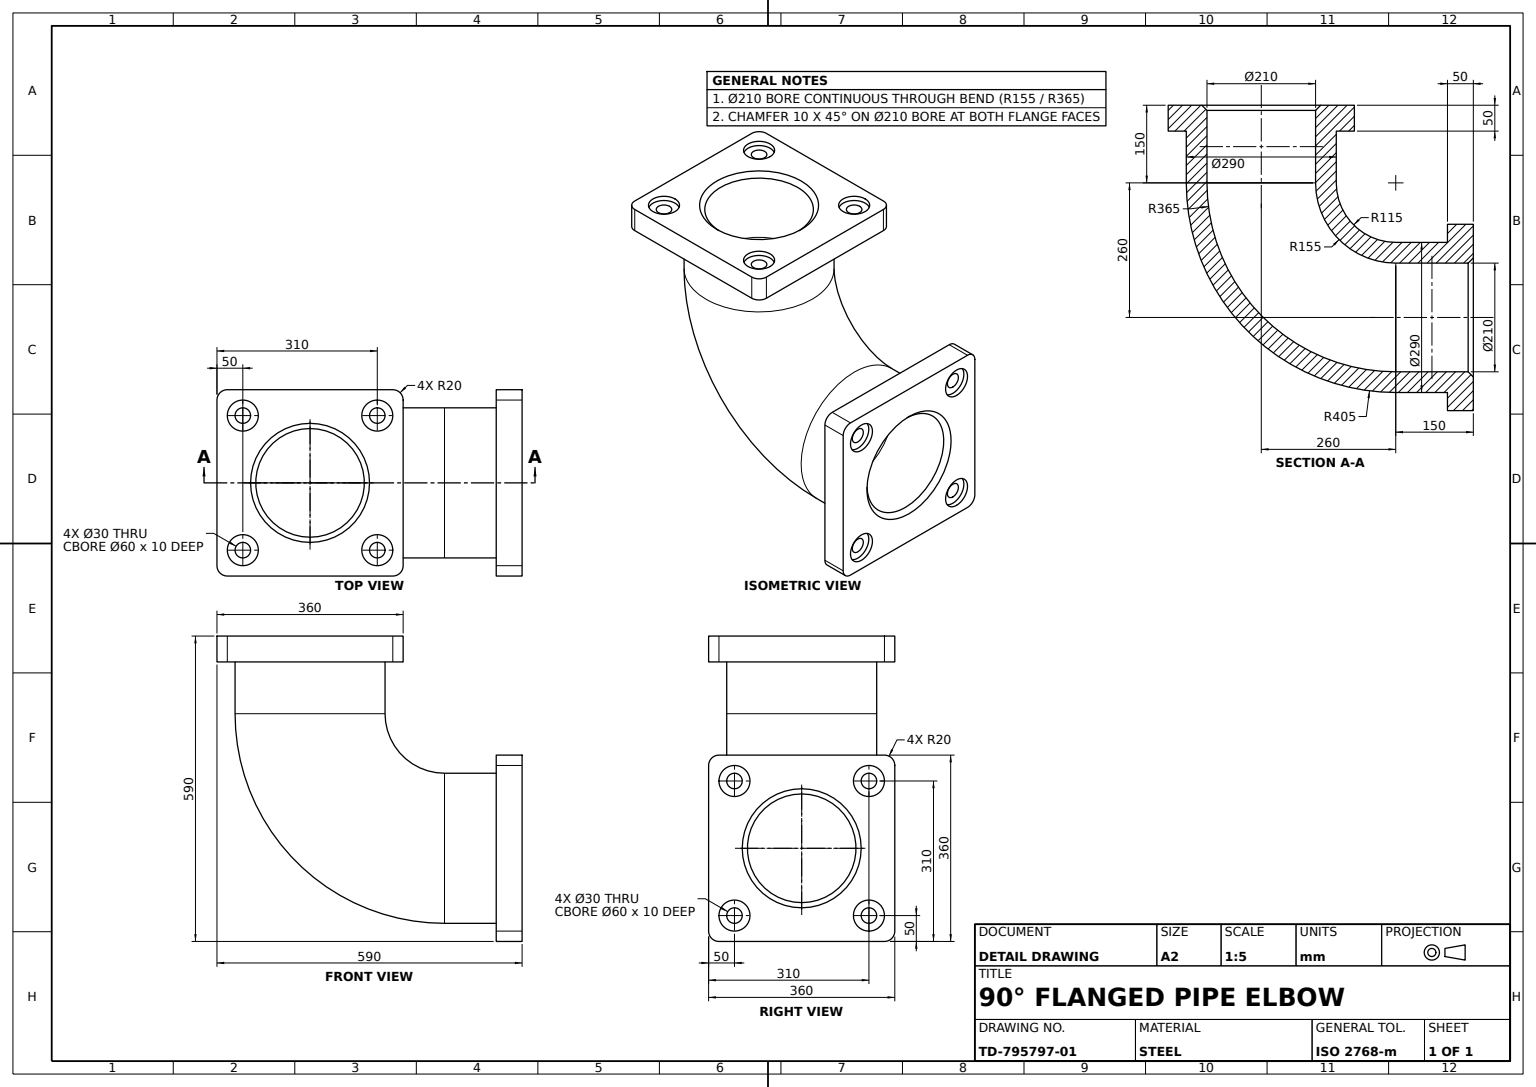
from build123d import *

# Parameters (mm, degrees)
PIPE_PROFILE_SKETCH_290_R           = 145
PIPE_PROFILE_SKETCH_290_R_2         = 105
FLANGE_START                        = -50
FLANGE_A_SKETCH_360X360_W           = 360
FLANGE_A_SKETCH_360X360_H           = 360
FLANGE_A_SKETCH_360X360_R           = 145
FLANGE_A_360X360X50_DEPTH           = 50
FLANGE_A_CORNER_FILLETS_R20_R       = 20
FLANGE_B_SKETCH_360X360_W           = 360
FLANGE_B_SKETCH_360X360_H           = 360
FLANGE_B_SKETCH_360X360_R           = 145
FLANGE_B_360X360X50_DEPTH           = 50
FLANGE_B_CORNER_FILLETS_R20_R       = 20
FLANGE_A_COUNTERBORE_SKETCH_60_R    = 30
FLANGE_A_COUNTERBORE_60X10_DEPTH    = 10
FLANGE_A_BOLT_HOLE_30_REACH         = 734.735
FLANGE_A_BOLT_HOLE_SKETCH_30_R      = 15
FLANGE_A_BOLT_HOLE_PATTERN_4X_COUNT = 4
FLANGE_B_COUNTERBORE_SKETCH_60_R    = 30
FLANGE_B_COUNTERBORE_60X10_DEPTH    = 10
FLANGE_B_BOLT_HOLE_30_REACH         = 848.699
FLANGE_B_BOLT_HOLE_SKETCH_30_R      = 15
FLANGE_B_BOLT_HOLE_PATTERN_4X_COUNT = 4
PIPE_EDGE_CHAMFER_10X45DEG_SIZE     = 10


with BuildPart() as part:
    # Elbow Pipe Sweep Wall 40: sweep along a path in Elbow Path Sketch
    with BuildLine(Plane.XY) as elbow_pipe_sweep_wall_40_path:
        Line((0, 0), (-150, 0))
        ThreePointArc((-150, 0), (-333.847763109, 76.152236891), (-410, 260))
        Line((-410, 260), (-410, 410))
    # Pipe Profile Sketch Ø290 → Elbow Pipe Sweep Wall 40 (sweep)
    with BuildSketch(Plane(origin=(0, 0, 0), x_dir=(0, 0, -1), z_dir=(1, 0, 0))):
        Circle(PIPE_PROFILE_SKETCH_290_R)
        Circle(PIPE_PROFILE_SKETCH_290_R_2, mode=Mode.SUBTRACT)
    sweep(path=elbow_pipe_sweep_wall_40_path.line)

    # Flange A Sketch 360x360 → Flange A 360x360x50 (add)
    with BuildSketch(Plane(origin=(0, 0, 0), x_dir=(0, 0, -1), z_dir=(1, 0, 0)).offset(FLANGE_START)):
        Rectangle(FLANGE_A_SKETCH_360X360_W, FLANGE_A_SKETCH_360X360_H)
        with Locations(Location((0, 0, 0), (0, 0, 270))):
            Circle(FLANGE_A_SKETCH_360X360_R, mode=Mode.SUBTRACT)
    extrude(amount=FLANGE_A_360X360X50_DEPTH)

    # Flange A Corner Fillets R20
    flange_a_corner_fillets_r20_edges = [part.edges().sort_by_distance(p)[0] for p in [
        (-25, 180, -180),
        (-25, -180, -180),
        (-25, -180, 180),
        (-25, 180, 180),
    ]]
    fillet(flange_a_corner_fillets_r20_edges, radius=FLANGE_A_CORNER_FILLETS_R20_R)

    # Flange B Sketch 360x360 → Flange B 360x360x50 (add)
    with BuildSketch(Plane(origin=(0, 410, 0), x_dir=(1, 0, 0), z_dir=(0, 1, 0))):
        with Locations((-410, 0)):
            Rectangle(FLANGE_B_SKETCH_360X360_W, FLANGE_B_SKETCH_360X360_H)
        with Locations(Location((-410, 0, 0), (0, 0, 180))):
            Circle(FLANGE_B_SKETCH_360X360_R, mode=Mode.SUBTRACT)
    extrude(amount=-FLANGE_B_360X360X50_DEPTH)

    # Flange B Corner Fillets R20
    flange_b_corner_fillets_r20_edges = [part.edges().sort_by_distance(p)[0] for p in [
        (-230, 385, -180),
        (-230, 385, 180),
        (-590, 385, 180),
        (-590, 385, -180),
    ]]
    fillet(flange_b_corner_fillets_r20_edges, radius=FLANGE_B_CORNER_FILLETS_R20_R)

    # Flange A Counterbore Sketch Ø60 → Flange A Counterbore Ø60x10 (cut)
    with BuildSketch(Plane(origin=(0, 0, 0), x_dir=(0, 0, -1), z_dir=(1, 0, 0))):
        with Locations((-130, 130)):
            Circle(FLANGE_A_COUNTERBORE_SKETCH_60_R)
    flange_a_counterbore_60x10 = extrude(amount=-FLANGE_A_COUNTERBORE_60X10_DEPTH, mode=Mode.SUBTRACT)

    # Flange A Bolt Hole Sketch Ø30 → Flange A Bolt Hole Ø30 (cut, up to next)
    with BuildSketch(Plane(origin=(-10, 0, 0), x_dir=(0, 0, -1), z_dir=(1, 0, 0)), mode=Mode.PRIVATE) as flange_a_bolt_hole_30_sk1:
        with Locations((-130, 130)):
            Circle(FLANGE_A_BOLT_HOLE_SKETCH_30_R)
    flange_a_bolt_hole_30_tool1 = extrude(flange_a_bolt_hole_30_sk1.sketch, amount=-FLANGE_A_BOLT_HOLE_30_REACH, mode=Mode.PRIVATE) & part.part
    flange_a_bolt_hole_30 = flange_a_bolt_hole_30_tool1.solids().sort_by_distance((-10, 130, 130))[0]
    add(flange_a_bolt_hole_30, mode=Mode.SUBTRACT)

    # Flange A Bolt Hole Pattern 4x: Flange A Counterbore Ø60x10, Flange A Bolt Hole Ø30 ×4 about axis
    flange_a_bolt_hole_pattern_4x_axis = Axis((0, 0, 0), (1, 0, 0))
    add([flange_a_counterbore_60x10.rotate(flange_a_bolt_hole_pattern_4x_axis, i * 360 / FLANGE_A_BOLT_HOLE_PATTERN_4X_COUNT) for i in range(1, FLANGE_A_BOLT_HOLE_PATTERN_4X_COUNT)], mode=Mode.SUBTRACT)
    add([flange_a_bolt_hole_30.rotate(flange_a_bolt_hole_pattern_4x_axis, i * 360 / FLANGE_A_BOLT_HOLE_PATTERN_4X_COUNT) for i in range(1, FLANGE_A_BOLT_HOLE_PATTERN_4X_COUNT)], mode=Mode.SUBTRACT)

    # Flange B Counterbore Sketch Ø60 → Flange B Counterbore Ø60x10 (cut)
    with BuildSketch(Plane(origin=(0, 410, 0), x_dir=(1, 0, 0), z_dir=(0, 1, 0))):
        with Locations(Location((-540, 130, 0), (0, 0, 180))):
            Circle(FLANGE_B_COUNTERBORE_SKETCH_60_R)
    flange_b_counterbore_60x10 = extrude(amount=-FLANGE_B_COUNTERBORE_60X10_DEPTH, mode=Mode.SUBTRACT)

    # Flange B Bolt Hole Sketch Ø30 → Flange B Bolt Hole Ø30 (cut, up to next)
    with BuildSketch(Plane(origin=(0, 400, 0), x_dir=(1, 0, 0), z_dir=(0, 1, 0)), mode=Mode.PRIVATE) as flange_b_bolt_hole_30_sk1:
        with Locations(Location((-540, 130, 0), (0, 0, 180))):
            Circle(FLANGE_B_BOLT_HOLE_SKETCH_30_R)
    flange_b_bolt_hole_30_tool1 = extrude(flange_b_bolt_hole_30_sk1.sketch, amount=-FLANGE_B_BOLT_HOLE_30_REACH, mode=Mode.PRIVATE) & part.part
    flange_b_bolt_hole_30 = flange_b_bolt_hole_30_tool1.solids().sort_by_distance((-540, 400, -130))[0]
    add(flange_b_bolt_hole_30, mode=Mode.SUBTRACT)

    # Flange B Bolt Hole Pattern 4x: Flange B Counterbore Ø60x10, Flange B Bolt Hole Ø30 ×4 about axis
    flange_b_bolt_hole_pattern_4x_axis = Axis((-410, 0, 0), (0, 1, 0))
    add([flange_b_counterbore_60x10.rotate(flange_b_bolt_hole_pattern_4x_axis, i * 360 / FLANGE_B_BOLT_HOLE_PATTERN_4X_COUNT) for i in range(1, FLANGE_B_BOLT_HOLE_PATTERN_4X_COUNT)], mode=Mode.SUBTRACT)
    add([flange_b_bolt_hole_30.rotate(flange_b_bolt_hole_pattern_4x_axis, i * 360 / FLANGE_B_BOLT_HOLE_PATTERN_4X_COUNT) for i in range(1, FLANGE_B_BOLT_HOLE_PATTERN_4X_COUNT)], mode=Mode.SUBTRACT)

    # Pipe Edge Chamfer 10x45deg
    pipe_edge_chamfer_10x45deg_edges = [part.edges().sort_by_distance(p)[0] for p in [
        (0, 0, 105),
        (-410, 410, 105),
    ]]
    chamfer(pipe_edge_chamfer_10x45deg_edges, length=PIPE_EDGE_CHAMFER_10X45DEG_SIZE)


solid = part.part
